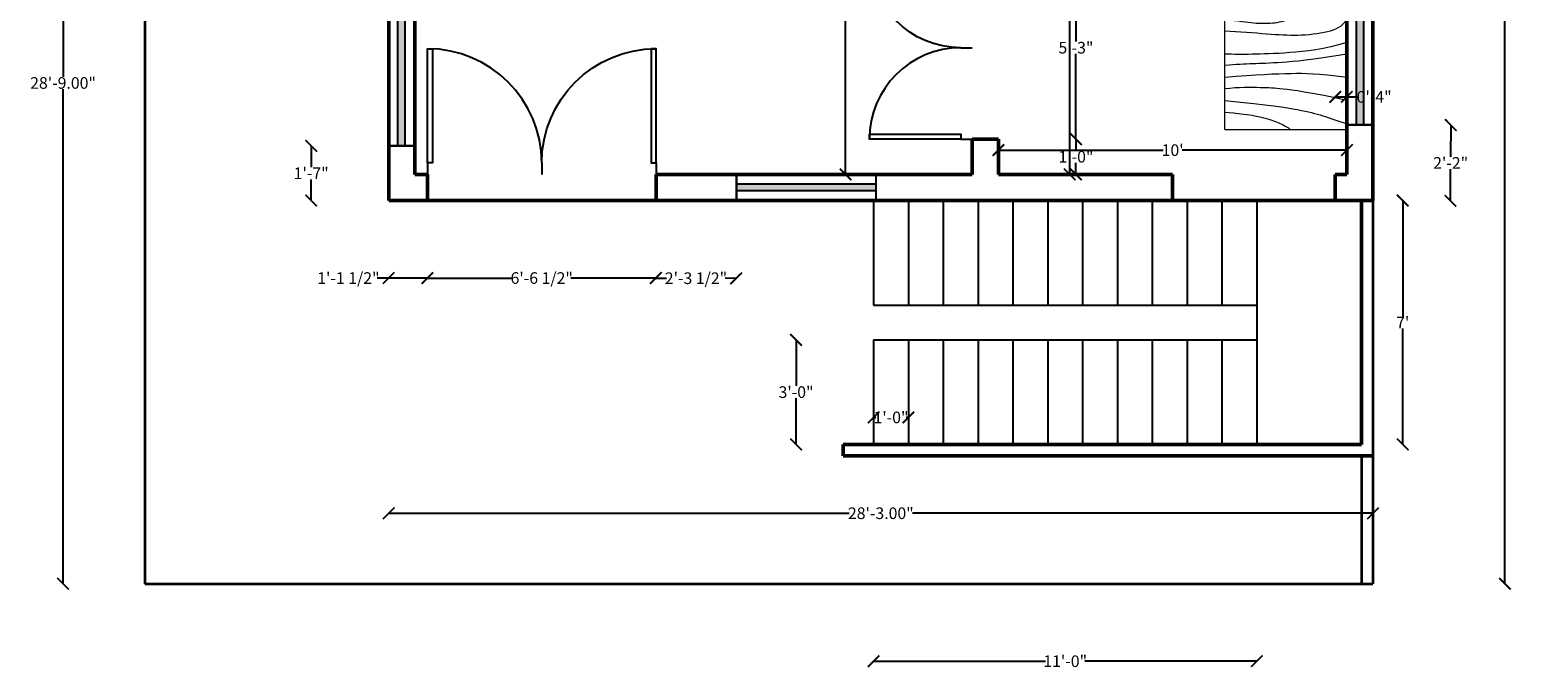
# Model space of a CAD drawing. Units: inches. Extents: x 2466 to 2986, y -30 to 527.
# Tile 1 of 5: x 2466 to 2986, y -30 to 190. Entities that reach past the tile are written whole.
import ezdxf

# ---------------------------------------------------------------- set-up
doc = ezdxf.new("R2010")
doc.units = ezdxf.units.IN
for name, color, linetype, lineweight in [('A-ANNO-DIMS', 2, 'Continuous', 18), ('A-GLAZ', 4, 'Continuous', 25), ('C-PROP', 40, 'Continuous', 35), ('doors', 3, 'Continuous', 25), ('furniture', 6, 'Continuous', 18), ('STAIRS', 1, 'Continuous', 25), ('walls', 40, 'Continuous', 50)]:
    doc.layers.add(name, color=color, linetype=linetype, lineweight=lineweight)
doc.styles.get("Standard").update_dxf_attribs({"font": 'arial.ttf'})
doc.dimstyles.get("Standard").update_dxf_attribs({"dimtxt": 4, "dimasz": 4, "dimexe": 0.18, "dimexo": 0.0625, "dimgap": 0.09, "dimtad": 0, "dimtih": 1, "dimtoh": 1, "dimzin": 0, "dimdsep": 46, "dimlunit": 3, "dimtxsty": 'Standard', "dimblk": 'ARCHTICK', "dimcen": 0.09, "dimse1": 1, "dimse2": 1, "dimclrd": 3, "dimclrt": 2, "dimadec": 0, "dimazin": 0, "dimtfac": 1, "dimtofl": 0, "dimtmove": 0, "dimatfit": 3, "dimfxl": 1, "dimtolj": 1, "dimtzin": 0, "dimarcsym": 0})

# ---------------------------------------------------------------- blocks, each defined once
blk = doc.blocks.new('*U5')
for p, q in [((0, 0), (0, -100)), ((1000, 0), (1000, -100))]:
    blk.add_line(p, q)
blk.add_lwpolyline([(0, 0), (0, 1000), (43.75, 1000), (43.75, 0)], close=True)
blk.add_arc((0, 0), 1000, 0, 90)
blk = doc.blocks.new('Table - Square Woodgrain 42 x 42 in.')
blk.add_line((0, -42), (42, -42))
for points in [[(0, -4), (1.704, -4.2172), (3.2358, -4.4188), (4.615, -4.604), (5.8615, -4.7721), (6.9951, -4.9224), (8.0357, -5.0541), (9.0031, -5.1667), (9.9171, -5.2594), (10.7951, -5.3316), (11.6445, -5.3836), (12.4702, -5.4157), (13.277, -5.4283), (14.0698, -5.4217), (14.8535, -5.3964), (15.6331, -5.3526), (16.4133, -5.2908), (17.1986, -5.2103), (17.9913, -5.1062), (18.793, -4.9727), (19.6056, -4.8038), (20.4307, -4.5937), (21.2701, -4.3365), (22.1256, -4.0262), (22.9989, -3.6571), (23.888, -3.2272), (24.7756, -2.7516), (25.6408, -2.2491), (26.4624, -1.7387), (27.2195, -1.2395), (27.891, -0.7703), (28.456, -0.3501), (28.8934, 0.002)], [(0, -42), (0, 0), (42, 0), (42, -42)], [(0, -8), (1.8203, -8.1001), (3.6741, -8.2149), (5.5411, -8.3408), (7.4011, -8.4741), (9.2339, -8.6112), (11.0193, -8.7484), (12.7371, -8.8821), (14.3671, -9.0086), (15.8954, -9.1246), (17.3337, -9.2278), (18.6997, -9.3159), (20.0116, -9.387), (21.2871, -9.4389), (22.5442, -9.4696), (23.8008, -9.477), (25.0749, -9.459), (26.3791, -9.4137), (27.7049, -9.3403), (29.0383, -9.2382), (30.3655, -9.1068), (31.6728, -8.9455), (32.9461, -8.7535), (34.1717, -8.5304), (35.3358, -8.2756), (36.4268, -7.9863), (37.443, -7.6521), (38.3849, -7.2603), (39.253, -6.7986), (40.048, -6.2542), (40.7705, -5.6147), (41.421, -4.8674), (42, -4)], [(42, -12), (39.1784, -12.8621), (36.4519, -13.5654), (33.8246, -14.1294), (31.3004, -14.5731), (28.8832, -14.9161), (26.577, -15.1775), (24.3858, -15.3768), (22.3136, -15.5332), (20.3622, -15.6632), (18.5254, -15.7718), (16.7947, -15.8612), (15.1618, -15.9338), (13.6183, -15.9916), (12.1558, -16.0369), (10.7659, -16.0718), (9.4403, -16.0987), (8.1703, -16.1191), (6.9461, -16.1325), (5.7577, -16.1377), (4.595, -16.1335), (3.4479, -16.1188), (2.3064, -16.0924), (1.1604, -16.0532), (0, -16)], [(42, -16), (37.6529, -16.7365), (33.8802, -17.329), (30.6179, -17.7961), (27.8015, -18.1561), (25.3668, -18.4275), (23.2497, -18.6288), (21.3859, -18.7785), (19.7111, -18.8949), (18.1693, -18.9939), (16.7375, -19.0795), (15.401, -19.1534), (14.1449, -19.217), (12.9544, -19.2717), (11.8148, -19.3191), (10.7113, -19.3606), (9.6291, -19.3976), (8.5534, -19.4323), (7.47, -19.4689), (6.3643, -19.5122), (5.222, -19.5672), (4.0288, -19.6386), (2.7703, -19.7313), (1.4321, -19.8501), (0, -20)], [(0, -24), (3.9243, -23.6805), (7.4766, -23.4138), (10.6891, -23.1954), (13.5943, -23.0205), (16.2247, -22.8847), (18.6125, -22.7832), (20.7903, -22.7116), (22.7903, -22.6651), (24.6563, -22.642), (26.4764, -22.6507), (28.35, -22.7024), (30.3766, -22.8084), (32.6555, -22.98), (35.2861, -23.2283), (38.3678, -23.5645), (42, -24)], [(42, -32), (37.392, -31.017), (33.4585, -30.2231), (30.1291, -29.5949), (27.3334, -29.109), (25.0009, -28.742), (23.0612, -28.4707), (21.4439, -28.2716), (20.0786, -28.1215), (18.8998, -28.0002), (17.8609, -27.9014), (16.9206, -27.8219), (16.0371, -27.7588), (15.1691, -27.709), (14.2748, -27.6693), (13.3128, -27.6368), (12.2415, -27.6083), (11.0295, -27.5824), (9.6867, -27.5643), (8.233, -27.5608), (6.6884, -27.5787), (5.0728, -27.6248), (3.4062, -27.7058), (1.7086, -27.8286), (0, -28)], [(0, -32), (5.4026, -32.5358), (9.9494, -33.019), (13.7424, -33.4553), (16.8834, -33.8505), (19.4743, -34.2106), (21.6171, -34.5413), (23.4136, -34.8486), (24.9657, -35.1382), (26.3614, -35.4156), (27.6332, -35.6841), (28.7995, -35.9467), (29.8788, -36.2064), (30.8897, -36.4661), (31.8507, -36.7288), (32.7802, -36.9973), (33.6968, -37.2747), (34.6175, -37.5635), (35.5531, -37.8651), (36.5128, -38.1805), (37.506, -38.5108), (38.5421, -38.8568), (39.6302, -39.2197), (40.7797, -39.6004), (42, -40)], [(0, -36), (3.0098, -36.2857), (5.5354, -36.5643), (7.6368, -36.8359), (9.374, -37.1009), (10.807, -37.3597), (11.9957, -37.6126), (13.0002, -37.8599), (13.8804, -38.102), (14.6874, -38.3393), (15.4365, -38.5729), (16.1338, -38.8041), (16.7858, -39.0341), (17.3987, -39.264), (17.9787, -39.4952), (18.5322, -39.7288), (19.0655, -39.9662), (19.5832, -40.2081), (20.0842, -40.4544), (20.5657, -40.7046), (21.0249, -40.9581), (21.459, -41.2144), (21.8653, -41.4731), (22.2409, -41.7335), (22.5831, -41.9951)]]:
    blk.add_lwpolyline(points)
blk = doc.blocks.new('*U18')
for p, q in [((0, 0), (0, -100)), ((800, 0), (800, -100))]:
    blk.add_line(p, q)
blk.add_lwpolyline([(0, 0), (0, 800), (43.75, 800), (43.75, 0)], close=True)
blk.add_arc((0, 0), 800, 0, 90)
blk = doc.blocks.new('_ArchTick')
at = {"color": 0, "linetype": 'ByBlock', "const_width": 0.15}
blk.add_lwpolyline([(-0.5, -0.5), (0.5, 0.5)], dxfattribs=at)
blk = doc.blocks.new('*D19')
at = {"layer": 'A-ANNO-DIMS', "color": 0, "lineweight": -2, "transparency": 16777216}
for p, q in [((2477.58, 344.8), (2477.58, 174.43)), ((2477.58, -0.2), (2477.58, 170.16))]:
    blk.add_line(p, q, dxfattribs=at)
at = {"layer": 'Defpoints', "color": 0, "transparency": 16777216}
for p in [(2477.58, 344.8), (2505.73, 344.8), (2505.73, -0.2)]:
    blk.add_point(p, dxfattribs=at)
at = {"layer": 'A-ANNO-DIMS', "color": 0, "lineweight": -2, "transparency": 16777216, "xscale": 4, "yscale": 4, "zscale": 4}
for p, rotation in [((2477.58, 344.8), 90), ((2477.58, -0.2), 270)]:
    blk.add_blockref('_ArchTick', p, dxfattribs=dict(at, rotation=rotation))
at = {"layer": 'A-ANNO-DIMS', "color": 0, "transparency": 16777216, "insert": (2477.58, 172.3), "char_height": 4, "attachment_point": 5}
blk.add_mtext('\\A1;28\'-9.00"', dxfattribs=at)
blk = doc.blocks.new('*D22')
at = {"layer": 'A-ANNO-DIMS', "color": 0, "lineweight": -2, "transparency": 16777216}
for p, q in [((2974.18, 494.8), (2974.18, 249.43)), ((2974.18, -0.2), (2974.18, 245.16))]:
    blk.add_line(p, q, dxfattribs=at)
at = {"layer": 'Defpoints', "color": 0, "transparency": 16777216}
for p in [(2928.73, 494.8), (2928.73, -0.2), (2974.18, -0.2)]:
    blk.add_point(p, dxfattribs=at)
at = {"layer": 'A-ANNO-DIMS', "color": 0, "lineweight": -2, "transparency": 16777216, "xscale": 4, "yscale": 4, "zscale": 4}
for p, rotation in [((2974.18, 494.8), 90), ((2974.18, -0.2), 270)]:
    blk.add_blockref('_ArchTick', p, dxfattribs=dict(at, rotation=rotation))
at = {"layer": 'A-ANNO-DIMS', "color": 0, "transparency": 16777216, "insert": (2974.18, 247.3), "char_height": 4, "attachment_point": 5}
blk.add_mtext('\\A1;41\'-3.00"', dxfattribs=at)
blk = doc.blocks.new('*D27')
at = {"layer": 'A-ANNO-DIMS', "color": 0, "lineweight": -2, "transparency": 16777216}
for p, q in [((2824.31, 272.8), (2824.31, 208.89)), ((2824.31, 140.8), (2824.31, 204.7))]:
    blk.add_line(p, q, dxfattribs=at)
at = {"layer": 'Defpoints', "color": 0, "transparency": 16777216}
for p in [(2799.73, 272.8), (2824.31, 272.8), (2799.73, 140.8)]:
    blk.add_point(p, dxfattribs=at)
at = {"layer": 'A-ANNO-DIMS', "color": 0, "lineweight": -2, "transparency": 16777216, "xscale": 4, "yscale": 4, "zscale": 4}
for p, rotation in [((2824.31, 272.8), 90), ((2824.31, 140.8), 270)]:
    blk.add_blockref('_ArchTick', p, dxfattribs=dict(at, rotation=rotation))
at = {"layer": 'A-ANNO-DIMS', "color": 0, "transparency": 16777216, "insert": (2824.31, 206.8), "char_height": 4, "attachment_point": 5}
blk.add_mtext("\\A1;11'", dxfattribs=at)
blk = doc.blocks.new('*D28')
at = {"layer": 'A-ANNO-DIMS', "color": 0, "lineweight": -2, "transparency": 16777216}
for p, q in [((2799.73, 149.17), (2856.43, 149.17)), ((2919.73, 149.17), (2863.02, 149.17))]:
    blk.add_line(p, q, dxfattribs=at)
at = {"layer": 'Defpoints', "color": 0, "transparency": 16777216}
for p in [(2919.73, 149.17), (2799.73, 140.8), (2919.73, 140.8)]:
    blk.add_point(p, dxfattribs=at)
at = {"layer": 'A-ANNO-DIMS', "color": 0, "lineweight": -2, "transparency": 16777216, "xscale": 4, "yscale": 4, "zscale": 4, "rotation": 180}
blk.add_blockref('_ArchTick', (2799.73, 149.17), dxfattribs=at)
at = {"layer": 'A-ANNO-DIMS', "color": 0, "lineweight": -2, "transparency": 16777216, "xscale": 4, "yscale": 4, "zscale": 4}
blk.add_blockref('_ArchTick', (2919.73, 149.17), dxfattribs=at)
at = {"layer": 'A-ANNO-DIMS', "color": 0, "transparency": 16777216, "insert": (2859.73, 149.17), "char_height": 4, "attachment_point": 5}
blk.add_mtext("\\A1;10'", dxfattribs=at)
blk = doc.blocks.new('*D33')
at = {"layer": 'A-ANNO-DIMS', "color": 0, "lineweight": -2, "transparency": 16777216}
for p, q in [((2938.97, 131.8), (2938.97, 91.89)), ((2938.97, 47.8), (2938.97, 87.71))]:
    blk.add_line(p, q, dxfattribs=at)
at = {"layer": 'Defpoints', "color": 0, "transparency": 16777216}
for p in [(2924.73, 131.8), (2924.73, 47.8), (2938.97, 47.8)]:
    blk.add_point(p, dxfattribs=at)
at = {"layer": 'A-ANNO-DIMS', "color": 0, "lineweight": -2, "transparency": 16777216, "xscale": 4, "yscale": 4, "zscale": 4}
for p, rotation in [((2938.97, 131.8), 90), ((2938.97, 47.8), 270)]:
    blk.add_blockref('_ArchTick', p, dxfattribs=dict(at, rotation=rotation))
at = {"layer": 'A-ANNO-DIMS', "color": 0, "transparency": 16777216, "insert": (2938.97, 89.8), "char_height": 4, "attachment_point": 5}
blk.add_mtext("\\A1;7'", dxfattribs=at)
blk = doc.blocks.new('*D34')
at = {"layer": 'A-ANNO-DIMS', "color": 0, "lineweight": -2, "transparency": 16777216}
for p, q in [((2589.73, 24.07), (2748.35, 24.07)), ((2928.73, 24.07), (2770.1, 24.07))]:
    blk.add_line(p, q, dxfattribs=at)
at = {"layer": 'Defpoints', "color": 0, "transparency": 16777216}
for p in [(2589.73, 131.8), (2928.73, 131.8), (2928.73, 24.07)]:
    blk.add_point(p, dxfattribs=at)
at = {"layer": 'A-ANNO-DIMS', "color": 0, "lineweight": -2, "transparency": 16777216, "xscale": 4, "yscale": 4, "zscale": 4, "rotation": 180}
blk.add_blockref('_ArchTick', (2589.73, 24.07), dxfattribs=at)
at = {"layer": 'A-ANNO-DIMS', "color": 0, "lineweight": -2, "transparency": 16777216, "xscale": 4, "yscale": 4, "zscale": 4}
blk.add_blockref('_ArchTick', (2928.73, 24.07), dxfattribs=at)
at = {"layer": 'A-ANNO-DIMS', "color": 0, "transparency": 16777216, "insert": (2759.23, 24.07), "char_height": 4, "attachment_point": 5}
blk.add_mtext('\\A1;28\'-3.00"', dxfattribs=at)
blk = doc.blocks.new('*D35')
at = {"layer": 'A-ANNO-DIMS', "color": 0, "lineweight": -2, "transparency": 16777216}
for p, q in [((2747.09, 344.8), (2747.09, 244.89)), ((2747.09, 140.8), (2747.09, 240.7))]:
    blk.add_line(p, q, dxfattribs=at)
at = {"layer": 'Defpoints', "color": 0, "transparency": 16777216}
for p in [(2776.87, 344.8), (2747.09, 140.8), (2776.87, 140.8)]:
    blk.add_point(p, dxfattribs=at)
at = {"layer": 'A-ANNO-DIMS', "color": 0, "lineweight": -2, "transparency": 16777216, "xscale": 4, "yscale": 4, "zscale": 4}
for p, rotation in [((2747.09, 344.8), 90), ((2747.09, 140.8), 270)]:
    blk.add_blockref('_ArchTick', p, dxfattribs=dict(at, rotation=rotation))
at = {"layer": 'A-ANNO-DIMS', "color": 0, "transparency": 16777216, "insert": (2747.09, 242.8), "char_height": 4, "attachment_point": 5}
blk.add_mtext("\\A1;17'", dxfattribs=at)
blk = doc.blocks.new('WIN-62_38IN')
h = blk.add_hatch(color=256)
h.dxf.hatch_style = 1
h.paths.add_polyline_path([(3.19, 0), (5.61, 0), (5.61, 62.38), (3.19, 62.38)])
for p, q in [((0, 62.38), (9, 62.38)), ((0, 0), (9, 0))]:
    blk.add_line(p, q)
for points in [[(0, 0), (0, 62.38), (9, 62.38), (9, 62.38), (9, 0)], [(3.19, 0), (3.19, 62.38), (5.61, 62.38), (5.61, 0)]]:
    blk.add_lwpolyline(points, close=True)
blk = doc.blocks.new('WIN-48IN')
h = blk.add_hatch(color=256)
h.dxf.hatch_style = 1
h.paths.add_polyline_path([(0, 5.81), (0, 3.39), (48, 3.39), (48, 5.81)])
for p, q in [((0, 9), (0, 0)), ((48, 9), (48, 0))]:
    blk.add_line(p, q)
for points in [[(0, 9), (48, 9), (48, 0), (0, 0)], [(0, 5.81), (48, 5.81), (48, 3.39), (0, 3.39)]]:
    blk.add_lwpolyline(points, close=True)
blk = doc.blocks.new('*D61')
at = {"layer": 'A-ANNO-DIMS', "color": 3, "lineweight": -2, "transparency": 16777216}
for p, q in [((2603.07, 105.1), (2632.36, 105.1)), ((2681.81, 105.1), (2652.51, 105.1))]:
    blk.add_line(p, q, dxfattribs=at)
at = {"layer": 'Defpoints', "color": 0, "transparency": 16777216}
for p in [(2603.07, 131.8), (2681.81, 131.8), (2603.07, 105.1)]:
    blk.add_point(p, dxfattribs=at)
at = {"layer": 'A-ANNO-DIMS', "color": 3, "lineweight": -2, "transparency": 16777216, "xscale": 4, "yscale": 4, "zscale": 4, "rotation": 180}
blk.add_blockref('_ArchTick', (2603.07, 105.1), dxfattribs=at)
at = {"layer": 'A-ANNO-DIMS', "color": 3, "lineweight": -2, "transparency": 16777216, "xscale": 4, "yscale": 4, "zscale": 4}
blk.add_blockref('_ArchTick', (2681.81, 105.1), dxfattribs=at)
at = {"layer": 'A-ANNO-DIMS', "color": 2, "transparency": 16777216, "insert": (2642.44, 105.1), "char_height": 4, "attachment_point": 5}
blk.add_mtext('\\A1;6\'-6 1/2"', dxfattribs=at)
blk = doc.blocks.new('*D64')
at = {"layer": 'A-ANNO-DIMS', "color": 3, "lineweight": -2, "transparency": 16777216}
for p, q in [((2826.43, 215.94), (2826.43, 186.57)), ((2826.43, 152.94), (2826.43, 182.31))]:
    blk.add_line(p, q, dxfattribs=at)
at = {"layer": 'Defpoints', "color": 0, "transparency": 16777216}
for p in [(2799.73, 215.94), (2799.73, 152.94), (2826.43, 152.94)]:
    blk.add_point(p, dxfattribs=at)
at = {"layer": 'A-ANNO-DIMS', "color": 3, "lineweight": -2, "transparency": 16777216, "xscale": 4, "yscale": 4, "zscale": 4}
for p, rotation in [((2826.43, 215.94), 90), ((2826.43, 152.94), 270)]:
    blk.add_blockref('_ArchTick', p, dxfattribs=dict(at, rotation=rotation))
at = {"layer": 'A-ANNO-DIMS', "color": 2, "transparency": 16777216, "insert": (2826.43, 184.44), "char_height": 4, "attachment_point": 5}
blk.add_mtext('\\A1;5\'-3"', dxfattribs=at)
blk = doc.blocks.new('*D66')
at = {"layer": 'A-ANNO-DIMS', "color": 3, "lineweight": -2, "transparency": 16777216}
for p, q in [((2756.73, -26.9), (2815.95, -26.9)), ((2888.73, -26.9), (2829.5, -26.9))]:
    blk.add_line(p, q, dxfattribs=at)
at = {"layer": 'Defpoints', "color": 0, "transparency": 16777216}
for p in [(2756.73, 47.8), (2888.73, 47.8), (2888.73, -26.9)]:
    blk.add_point(p, dxfattribs=at)
at = {"layer": 'A-ANNO-DIMS', "color": 3, "lineweight": -2, "transparency": 16777216, "xscale": 4, "yscale": 4, "zscale": 4, "rotation": 180}
blk.add_blockref('_ArchTick', (2756.73, -26.9), dxfattribs=at)
at = {"layer": 'A-ANNO-DIMS', "color": 3, "lineweight": -2, "transparency": 16777216, "xscale": 4, "yscale": 4, "zscale": 4}
blk.add_blockref('_ArchTick', (2888.73, -26.9), dxfattribs=at)
at = {"layer": 'A-ANNO-DIMS', "color": 2, "transparency": 16777216, "insert": (2822.73, -26.9), "char_height": 4, "attachment_point": 5}
blk.add_mtext('\\A1;11\'-0"', dxfattribs=at)
blk = doc.blocks.new('*D67')
at = {"layer": 'A-ANNO-DIMS', "color": 3, "lineweight": -2, "transparency": 16777216}
for p, q in [((2888.73, 521.5), (2901.32, 521.5)), ((2924.73, 521.5), (2912.13, 521.5))]:
    blk.add_line(p, q, dxfattribs=at)
at = {"layer": 'Defpoints', "color": 0, "transparency": 16777216}
for p in [(2924.73, 521.5), (2888.73, 47.8), (2924.73, 47.8)]:
    blk.add_point(p, dxfattribs=at)
at = {"layer": 'A-ANNO-DIMS', "color": 3, "lineweight": -2, "transparency": 16777216, "xscale": 4, "yscale": 4, "zscale": 4, "rotation": 180}
blk.add_blockref('_ArchTick', (2888.73, 521.5), dxfattribs=at)
at = {"layer": 'A-ANNO-DIMS', "color": 3, "lineweight": -2, "transparency": 16777216, "xscale": 4, "yscale": 4, "zscale": 4}
blk.add_blockref('_ArchTick', (2924.73, 521.5), dxfattribs=at)
at = {"layer": 'A-ANNO-DIMS', "color": 2, "transparency": 16777216, "insert": (2906.73, 521.5), "char_height": 4, "attachment_point": 5}
blk.add_mtext('\\A1;3\'-0"', dxfattribs=at)
blk = doc.blocks.new('*D68')
at = {"layer": 'A-ANNO-DIMS', "color": 3, "lineweight": -2, "transparency": 16777216}
for p, q in [((2730.03, 83.8), (2730.03, 67.93)), ((2730.03, 47.8), (2730.03, 63.66))]:
    blk.add_line(p, q, dxfattribs=at)
at = {"layer": 'Defpoints', "color": 0, "transparency": 16777216}
for p in [(2730.03, 83.8), (2756.73, 83.8), (2756.73, 47.8)]:
    blk.add_point(p, dxfattribs=at)
at = {"layer": 'A-ANNO-DIMS', "color": 3, "lineweight": -2, "transparency": 16777216, "xscale": 4, "yscale": 4, "zscale": 4}
for p, rotation in [((2730.03, 83.8), 90), ((2730.03, 47.8), 270)]:
    blk.add_blockref('_ArchTick', p, dxfattribs=dict(at, rotation=rotation))
at = {"layer": 'A-ANNO-DIMS', "color": 2, "transparency": 16777216, "insert": (2730.03, 65.8), "char_height": 4, "attachment_point": 5}
blk.add_mtext('\\A1;3\'-0"', dxfattribs=at)
blk = doc.blocks.new('*D70')
at = {"layer": 'A-ANNO-DIMS', "color": 3, "lineweight": -2, "transparency": 16777216}
for p, q in [((2859.73, 521.5), (2882.24, 521.5)), ((2915.73, 521.5), (2893.21, 521.5))]:
    blk.add_line(p, q, dxfattribs=at)
at = {"layer": 'Defpoints', "color": 0, "transparency": 16777216}
for p in [(2915.73, 521.5), (2859.73, 140.8), (2915.73, 140.8)]:
    blk.add_point(p, dxfattribs=at)
at = {"layer": 'A-ANNO-DIMS', "color": 3, "lineweight": -2, "transparency": 16777216, "xscale": 4, "yscale": 4, "zscale": 4, "rotation": 180}
blk.add_blockref('_ArchTick', (2859.73, 521.5), dxfattribs=at)
at = {"layer": 'A-ANNO-DIMS', "color": 3, "lineweight": -2, "transparency": 16777216, "xscale": 4, "yscale": 4, "zscale": 4}
blk.add_blockref('_ArchTick', (2915.73, 521.5), dxfattribs=at)
at = {"layer": 'A-ANNO-DIMS', "color": 2, "transparency": 16777216, "insert": (2887.73, 521.5), "char_height": 4, "attachment_point": 5}
blk.add_mtext('\\A1;4\'-8"', dxfattribs=at)
blk = doc.blocks.new('*D76')
at = {"layer": 'A-ANNO-DIMS', "color": 3, "lineweight": -2, "transparency": 16777216}
for p, q in [((2563.03, 150.61), (2563.03, 143.3)), ((2563.03, 131.8), (2563.03, 139.1))]:
    blk.add_line(p, q, dxfattribs=at)
at = {"layer": 'Defpoints', "color": 0, "transparency": 16777216}
for p in [(2563.03, 150.61), (2589.73, 150.61), (2589.73, 131.8)]:
    blk.add_point(p, dxfattribs=at)
at = {"layer": 'A-ANNO-DIMS', "color": 3, "lineweight": -2, "transparency": 16777216, "xscale": 4, "yscale": 4, "zscale": 4}
for p, rotation in [((2563.03, 150.61), 90), ((2563.03, 131.8), 270)]:
    blk.add_blockref('_ArchTick', p, dxfattribs=dict(at, rotation=rotation))
at = {"layer": 'A-ANNO-DIMS', "color": 2, "transparency": 16777216, "insert": (2563.03, 141.2), "char_height": 4, "attachment_point": 5}
blk.add_mtext('\\A1;1\'-7"', dxfattribs=at)
blk = doc.blocks.new('*D78')
at = {"layer": 'A-ANNO-DIMS', "color": 3, "lineweight": -2, "transparency": 16777216}
for p, q in [((2955.53, 157.8), (2955.48, 146.85)), ((2955.43, 131.69), (2955.47, 142.65))]:
    blk.add_line(p, q, dxfattribs=at)
at = {"layer": 'Defpoints', "color": 0, "transparency": 16777216}
for p in [(2928.83, 157.91), (2928.73, 131.8), (2955.43, 131.69)]:
    blk.add_point(p, dxfattribs=at)
at = {"layer": 'A-ANNO-DIMS', "color": 3, "lineweight": -2, "transparency": 16777216, "xscale": 4, "yscale": 4, "zscale": 4}
for p, rotation in [((2955.53, 157.8), 89.77598039140506), ((2955.43, 131.69), 269.7759803914051)]:
    blk.add_blockref('_ArchTick', p, dxfattribs=dict(at, rotation=rotation))
at = {"layer": 'A-ANNO-DIMS', "color": 2, "transparency": 16777216, "insert": (2955.48, 144.75), "char_height": 4, "attachment_point": 5}
blk.add_mtext('\\A1;2\'-2"', dxfattribs=at)
blk = doc.blocks.new('*D79')
at = {"layer": 'A-ANNO-DIMS', "color": 3, "lineweight": -2, "transparency": 16777216}
for p, q in [((2681.71, 105.1), (2685.46, 105.08)), ((2709.41, 104.99), (2705.66, 105.01))]:
    blk.add_line(p, q, dxfattribs=at)
at = {"layer": 'Defpoints', "color": 0, "transparency": 16777216}
for p in [(2681.81, 131.8), (2709.51, 131.69), (2681.71, 105.1)]:
    blk.add_point(p, dxfattribs=at)
at = {"layer": 'A-ANNO-DIMS', "color": 3, "lineweight": -2, "transparency": 16777216, "xscale": 4, "yscale": 4, "zscale": 4}
for p, rotation in [((2681.71, 105.1), 179.7888485670851), ((2709.41, 104.99), 359.7888485670852)]:
    blk.add_blockref('_ArchTick', p, dxfattribs=dict(at, rotation=rotation))
at = {"layer": 'A-ANNO-DIMS', "color": 2, "transparency": 16777216, "insert": (2695.56, 105.04), "char_height": 4, "attachment_point": 5}
blk.add_mtext('\\A1;2\'-3 1/2"', dxfattribs=at)
blk = doc.blocks.new('*D80')
at = {"layer": 'A-ANNO-DIMS', "color": 3, "lineweight": -2, "transparency": 16777216}
for p, q in [((2756.73, 57.1), (2757.51, 57.1)), ((2768.73, 57.1), (2767.94, 57.1))]:
    blk.add_line(p, q, dxfattribs=at)
at = {"layer": 'Defpoints', "color": 0, "transparency": 16777216}
for p in [(2756.73, 83.8), (2768.73, 83.8), (2756.73, 57.1)]:
    blk.add_point(p, dxfattribs=at)
at = {"layer": 'A-ANNO-DIMS', "color": 3, "lineweight": -2, "transparency": 16777216, "xscale": 4, "yscale": 4, "zscale": 4, "rotation": 180}
blk.add_blockref('_ArchTick', (2756.73, 57.1), dxfattribs=at)
at = {"layer": 'A-ANNO-DIMS', "color": 3, "lineweight": -2, "transparency": 16777216, "xscale": 4, "yscale": 4, "zscale": 4}
blk.add_blockref('_ArchTick', (2768.73, 57.1), dxfattribs=at)
at = {"layer": 'A-ANNO-DIMS', "color": 2, "transparency": 16777216, "insert": (2762.73, 57.1), "char_height": 4, "attachment_point": 5}
blk.add_mtext('\\A1;1\'-0"', dxfattribs=at)
blk = doc.blocks.new('*D81')
at = {"layer": 'A-ANNO-DIMS', "color": 3, "lineweight": -2, "transparency": 16777216}
for p, q in [((2589.73, 105.1), (2585.73, 105.1)), ((2603.07, 105.1), (2589.73, 105.1))]:
    blk.add_line(p, q, dxfattribs=at)
at = {"layer": 'Defpoints', "color": 0, "transparency": 16777216}
for p in [(2589.73, 131.8), (2603.07, 131.8), (2589.73, 105.1)]:
    blk.add_point(p, dxfattribs=at)
at = {"layer": 'A-ANNO-DIMS', "color": 3, "lineweight": -2, "transparency": 16777216, "xscale": 4, "yscale": 4, "zscale": 4, "rotation": 180}
blk.add_blockref('_ArchTick', (2589.73, 105.1), dxfattribs=at)
at = {"layer": 'A-ANNO-DIMS', "color": 3, "lineweight": -2, "transparency": 16777216, "xscale": 4, "yscale": 4, "zscale": 4}
blk.add_blockref('_ArchTick', (2603.07, 105.1), dxfattribs=at)
at = {"layer": 'A-ANNO-DIMS', "color": 2, "transparency": 16777216, "insert": (2575.85, 105.1), "char_height": 4, "attachment_point": 5}
blk.add_mtext('\\A1;1\'-1 1/2"', dxfattribs=at)
blk = doc.blocks.new('*D85')
at = {"layer": 'A-ANNO-DIMS', "color": 3, "lineweight": -2, "transparency": 16777216}
for p, q in [((2826.43, 152.94), (2826.43, 149)), ((2826.43, 140.8), (2826.43, 144.74))]:
    blk.add_line(p, q, dxfattribs=at)
at = {"layer": 'Defpoints', "color": 0, "transparency": 16777216}
for p in [(2799.73, 152.94), (2799.73, 140.8), (2826.43, 140.8)]:
    blk.add_point(p, dxfattribs=at)
at = {"layer": 'A-ANNO-DIMS', "color": 3, "lineweight": -2, "transparency": 16777216, "xscale": 4, "yscale": 4, "zscale": 4}
for p, rotation in [((2826.43, 152.94), 90), ((2826.43, 140.8), 270)]:
    blk.add_blockref('_ArchTick', p, dxfattribs=dict(at, rotation=rotation))
at = {"layer": 'A-ANNO-DIMS', "color": 2, "transparency": 16777216, "insert": (2826.43, 146.87), "char_height": 4, "attachment_point": 5}
blk.add_mtext('\\A1;1\'-0"', dxfattribs=at)
blk = doc.blocks.new('*D88')
at = {"layer": 'A-ANNO-DIMS', "color": 3, "lineweight": -2, "transparency": 16777216}
for p, q in [((2915.73, 167.5), (2919.73, 167.5)), ((2919.73, 167.5), (2923.73, 167.5))]:
    blk.add_line(p, q, dxfattribs=at)
at = {"layer": 'Defpoints', "color": 0, "transparency": 16777216}
for p in [(2919.73, 167.5), (2915.73, 140.8), (2919.73, 140.8)]:
    blk.add_point(p, dxfattribs=at)
at = {"layer": 'A-ANNO-DIMS', "color": 3, "lineweight": -2, "transparency": 16777216, "xscale": 4, "yscale": 4, "zscale": 4, "rotation": 180}
blk.add_blockref('_ArchTick', (2915.73, 167.5), dxfattribs=at)
at = {"layer": 'A-ANNO-DIMS', "color": 3, "lineweight": -2, "transparency": 16777216, "xscale": 4, "yscale": 4, "zscale": 4}
blk.add_blockref('_ArchTick', (2919.73, 167.5), dxfattribs=at)
at = {"layer": 'A-ANNO-DIMS', "color": 2, "transparency": 16777216, "insert": (2929.13, 167.5), "char_height": 4, "attachment_point": 5}
blk.add_mtext('\\A1;0\'-4"', dxfattribs=at)

msp = doc.modelspace()

# ---------------------------------------------------------------- linework, layer by layer
at = {"layer": 'C-PROP'}
for p, q in [((2505.725, 494.795), (2505.725, -0.205)), ((2928.725, 131.795), (2928.725, -0.205)), ((2924.725, 43.795), (2924.725, -0.205)), ((2505.725, -0.205), (2928.725, -0.205))]:
    msp.add_line(p, q, dxfattribs=at)
at = {"layer": 'STAIRS'}
for p, q in [((2756.725, 131.795), (2756.725, 95.795)), ((2768.725, 131.795), (2768.725, 95.795)), ((2780.725, 131.795), (2780.725, 95.795)), ((2792.725, 131.795), (2792.725, 95.795)), ((2804.725, 131.795), (2804.725, 95.795)), ((2816.725, 131.795), (2816.725, 95.795)), ((2828.725, 131.795), (2828.725, 95.795)), ((2840.725, 131.795), (2840.725, 95.795)), ((2852.725, 131.795), (2852.725, 95.795)), ((2864.725, 131.795), (2864.725, 95.795)), ((2876.725, 131.795), (2876.725, 95.795)), ((2888.725, 131.795), (2888.725, 83.795)), ((2756.725, 95.795), (2888.725, 95.795)), ((2756.725, 83.795), (2888.725, 83.795)), ((2756.725, 83.795), (2756.725, 47.795)), ((2768.725, 83.795), (2768.725, 47.795)), ((2780.725, 83.795), (2780.725, 47.795)), ((2792.725, 83.795), (2792.725, 47.795)), ((2804.725, 83.795), (2804.725, 47.795)), ((2816.725, 83.795), (2816.725, 47.795)), ((2828.725, 83.795), (2828.725, 47.795)), ((2840.725, 83.795), (2840.725, 47.795)), ((2852.725, 83.795), (2852.725, 47.795)), ((2864.725, 83.795), (2864.725, 47.795)), ((2876.725, 83.795), (2876.725, 47.795)), ((2888.725, 83.795), (2888.725, 47.795))]:
    msp.add_line(p, q, dxfattribs=at)
at = {"layer": 'walls'}
for p, q in [((2928.725, 494.795), (2928.725, 131.795)), ((2589.725, 344.795), (2589.725, 131.795)), ((2598.725, 344.795), (2598.725, 140.795)), ((2919.725, 272.795), (2919.725, 140.795)), ((2799.725, 152.944), (2790.725, 152.944)), ((2790.725, 152.944), (2790.725, 140.795)), ((2799.725, 152.944), (2799.725, 140.795)), ((2598.725, 140.795), (2603.066, 140.795)), ((2603.066, 140.795), (2603.066, 131.795)), ((2681.806, 140.795), (2790.725, 140.795)), ((2681.806, 140.795), (2681.806, 131.795)), ((2799.725, 140.795), (2859.725, 140.795)), ((2859.725, 140.795), (2859.725, 131.795)), ((2919.725, 140.795), (2915.725, 140.795)), ((2915.725, 140.795), (2915.725, 131.795)), ((2589.725, 131.795), (2928.725, 131.795)), ((2924.725, 131.795), (2924.725, 47.795)), ((2746.205, 47.795), (2924.725, 47.795)), ((2746.205, 43.795), (2746.205, 47.795)), ((2746.205, 43.795), (2928.725, 43.795))]:
    msp.add_line(p, q, dxfattribs=at)

# ---------------------------------------------------------------- block references
at = {"layer": 'A-GLAZ'}
for name, p in [('WIN-62_38IN', (2919.828, 157.909)), ('WIN-62_38IN', (2589.725, 150.606)), ('WIN-48IN', (2709.511, 131.693))]:
    msp.add_blockref(name, p, dxfattribs=at)
at = {"layer": 'doors', "yscale": 0.0393700787401575, "zscale": 0.0393700787401575}
for name, p, xscale, rotation in [('*U18', (2786.788, 215.936), -0.0393700787401575, 90), ('*U5', (2681.806, 144.732), -0.0393700787401575, 359.9999999999986), ('*U18', (2786.788, 152.944), 0.0393700787401575, 90)]:
    msp.add_blockref(name, p, dxfattribs=dict(at, xscale=xscale, rotation=rotation))
at = {"layer": 'doors', "xscale": 0.0393700787401575, "yscale": 0.0393700787401575, "zscale": 0.0393700787401575}
msp.add_blockref('*U5', (2603.066, 144.732), dxfattribs=at)
at = {"layer": 'furniture'}
msp.add_blockref('Table - Square Woodgrain 42 x 42 in.', (2877.725, 198.274), dxfattribs=at)

# ---------------------------------------------------------------- dimensions: what is measured, and where the dimension line sits
at = {"layer": 'A-ANNO-DIMS'}
for base, p1, p2, override, picture, middle in [((2915.725, 521.495), (2859.725, 140.795), (2915.725, 140.795), {"dimdec": 1, "dimlfac": 1, "dimrnd": 0, "dimzin": 1, "dimdsep": 46, "dimlunit": 4, "dimfrac": 2}, '*D70', (2887.725, 521.495)), ((2924.725, 521.495), (2888.725, 47.795), (2924.725, 47.795), {"dimdec": 1, "dimlfac": 1, "dimrnd": 0, "dimzin": 1, "dimdsep": 46, "dimlunit": 4, "dimfrac": 2}, '*D67', (2906.725, 521.495)), ((2919.725, 167.495), (2915.725, 140.795), (2919.725, 140.795), {"dimdec": 1, "dimlfac": 1, "dimrnd": 0, "dimzin": 1, "dimdsep": 46, "dimlunit": 4, "dimfrac": 2}, '*D88', (2929.132, 167.495)), ((2919.725, 149.174), (2799.725, 140.795), (2919.725, 140.795), {"dimclrd": 0, "dimclre": 0, "dimclrt": 0}, '*D28', (2859.725, 149.174)), ((2928.725, 24.065), (2589.725, 131.795), (2928.725, 131.795), {"dimclrd": 0, "dimclre": 0, "dimclrt": 0}, '*D34', (2759.225, 24.065)), ((2888.725, -26.905), (2756.725, 47.795), (2888.725, 47.795), {"dimdec": 1, "dimlfac": 1, "dimrnd": 0, "dimzin": 1, "dimdsep": 46, "dimlunit": 4, "dimfrac": 2}, '*D66', (2822.725, -26.905))]:
    dim = msp.add_linear_dim(base=base, p1=p1, p2=p2, dimstyle='Standard', override=override, dxfattribs=at)
    dim.commit()
    dim.dimension.update_dxf_attribs({"geometry": picture, "text_midpoint": middle})
for base, p1, p2, angle, override, picture, middle in [((2974.184, -0.205), (2928.725, 494.795), (2928.725, -0.205), 90, {"dimclrd": 0, "dimclre": 0, "dimclrt": 0}, '*D22', (2974.184, 247.295)), ((2477.576, 344.795), (2505.725, -0.205), (2505.725, 344.795), 90, {"dimclrd": 0, "dimclre": 0, "dimclrt": 0}, '*D19', (2477.576, 172.295)), ((2747.088, 140.795), (2776.871, 344.795), (2776.871, 140.795), 90, {"dimclrd": 0, "dimclre": 0, "dimclrt": 0}, '*D35', (2747.088, 242.795)), ((2824.314, 272.795), (2799.725, 140.795), (2799.725, 272.795), 90, {"dimclrd": 0, "dimclre": 0, "dimclrt": 0}, '*D27', (2824.314, 206.795)), ((2826.425, 152.944), (2799.725, 215.936), (2799.725, 152.944), 270, {"dimdec": 1, "dimlfac": 1, "dimrnd": 0, "dimzin": 1, "dimdsep": 46, "dimlunit": 4, "dimfrac": 2}, '*D64', (2826.425, 184.44)), ((2955.425, 131.691), (2928.828, 157.909), (2928.725, 131.795), 269.77598, {"dimdec": 1, "dimlfac": 1, "dimrnd": 0, "dimzin": 1, "dimdsep": 46, "dimlunit": 4, "dimfrac": 2}, '*D78', (2955.476, 144.748)), ((2563.025, 150.606), (2589.725, 131.795), (2589.725, 150.606), 90, {"dimdec": 1, "dimlfac": 1, "dimrnd": 0, "dimzin": 1, "dimdsep": 46, "dimlunit": 4, "dimfrac": 2}, '*D76', (2563.025, 141.201)), ((2826.425, 140.795), (2799.725, 152.944), (2799.725, 140.795), 270, {"dimdec": 1, "dimlfac": 1, "dimrnd": 0, "dimzin": 1, "dimdsep": 46, "dimlunit": 4, "dimfrac": 2}, '*D85', (2826.425, 146.87)), ((2589.725, 105.095), (2603.066, 131.795), (2589.725, 131.795), 180, {"dimdec": 1, "dimlfac": 1, "dimrnd": 0, "dimzin": 1, "dimdsep": 46, "dimlunit": 4, "dimfrac": 2}, '*D81', (2575.847, 105.095)), ((2603.066, 105.095), (2681.806, 131.795), (2603.066, 131.795), 180, {"dimdec": 1, "dimlfac": 1, "dimrnd": 0, "dimzin": 1, "dimdsep": 46, "dimlunit": 4, "dimfrac": 2}, '*D61', (2642.436, 105.095)), ((2681.708, 105.096), (2709.511, 131.693), (2681.806, 131.795), 179.78885, {"dimdec": 1, "dimlfac": 1, "dimrnd": 0, "dimzin": 1, "dimdsep": 46, "dimlunit": 4, "dimfrac": 2}, '*D79', (2695.56, 105.045)), ((2938.971, 47.795), (2924.725, 131.795), (2924.725, 47.795), 90, {"dimclrd": 0, "dimclre": 0, "dimclrt": 0}, '*D33', (2938.971, 89.795)), ((2730.025, 83.795), (2756.725, 47.795), (2756.725, 83.795), 90, {"dimdec": 1, "dimlfac": 1, "dimrnd": 0, "dimzin": 1, "dimdsep": 46, "dimlunit": 4, "dimfrac": 2}, '*D68', (2730.025, 65.795)), ((2756.725, 57.095), (2768.725, 83.795), (2756.725, 83.795), 180, {"dimdec": 1, "dimlfac": 1, "dimrnd": 0, "dimzin": 1, "dimdsep": 46, "dimlunit": 4, "dimfrac": 2}, '*D80', (2762.725, 57.095))]:
    dim = msp.add_linear_dim(base=base, p1=p1, p2=p2, angle=angle, dimstyle='Standard', override=override, dxfattribs=at)
    dim.commit()
    dim.dimension.update_dxf_attribs({"geometry": picture, "text_midpoint": middle})

doc.saveas('drawing.dxf')
